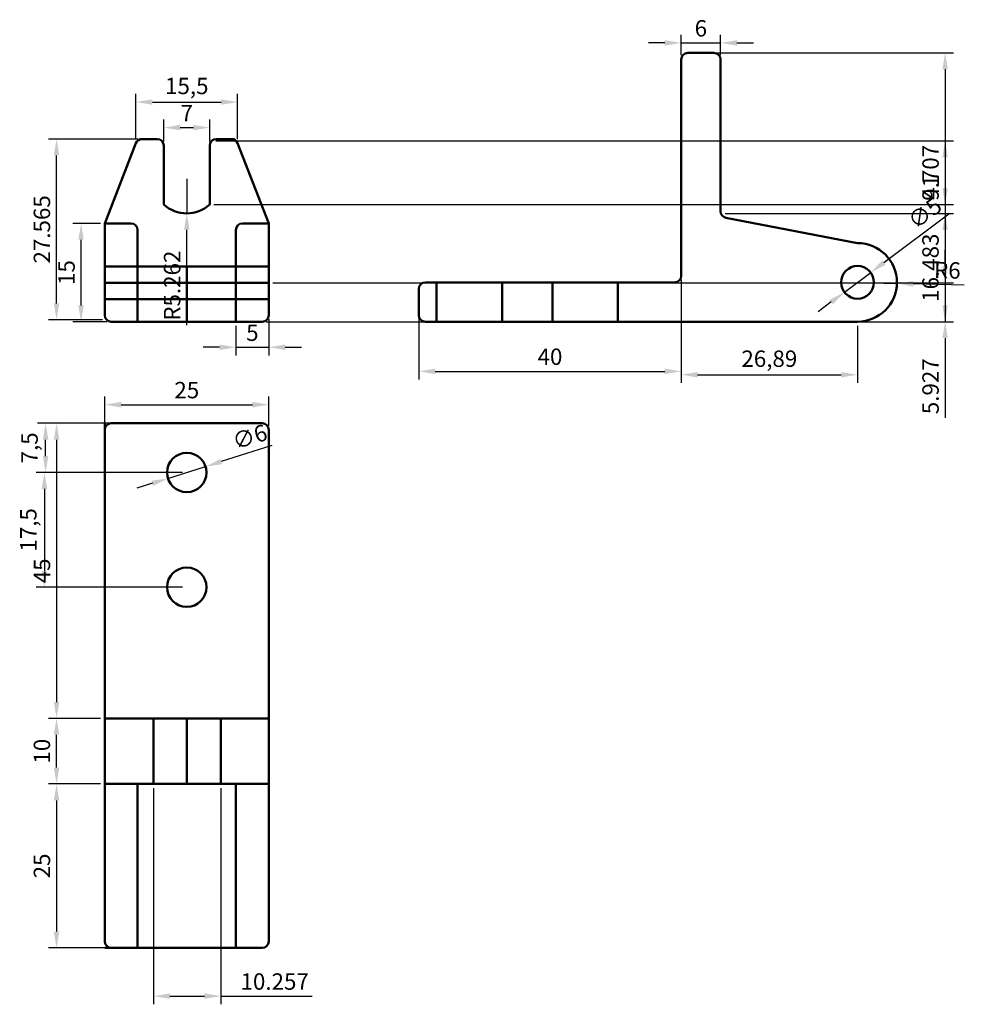
# Model space of a CAD drawing. Units: millimetres. Extents: x 2189 to 2333, y 2094 to 2245.
import ezdxf

# ---------------------------------------------------------------- set-up
doc = ezdxf.new("R2010")
doc.units = ezdxf.units.MM
doc.layers.add('M-DIMS', color=2, linetype='Continuous', lineweight=25)
doc.layers.add('M-OUTL', color=7, linetype='Continuous', lineweight=50)
doc.styles.get("Standard").update_dxf_attribs({"font": 'arial.ttf'})
doc.dimstyles.new('ISO-25', dxfattribs={"dimtxt": 2.5, "dimasz": 2.5, "dimexe": 1.25, "dimexo": 0.625, "dimtad": 1, "dimtxsty": 'Standard', "dimcen": 2.5, "dimadec": 0, "dimazin": 0, "dimtfac": 1, "dimtmove": 0, "dimatfit": 3, "dimfxl": 1, "dimarcsym": 0})

# ---------------------------------------------------------------- blocks, each defined once
blk = doc.blocks.new('*D1')
at = {"layer": 'Defpoints', "color": 0, "transparency": 16777216}
for p in [(2214.95, 2175.49), (2193.25, 2157.99), (2214.95, 2157.99)]:
    blk.add_point(p, dxfattribs=at)
at = {"layer": 'M-DIMS', "color": 0, "lineweight": -2, "transparency": 16777216}
for p, q in [((2214.32, 2175.49), (2192, 2175.49)), ((2193.25, 2172.99), (2193.25, 2160.49)), ((2214.32, 2157.99), (2192, 2157.99))]:
    blk.add_line(p, q, dxfattribs=at)
at = {"layer": 'M-DIMS', "color": 0, "transparency": 16777216}
for points in [[(2192.83, 2172.99), (2193.66, 2172.99), (2193.25, 2175.49)], [(2192.83, 2160.49), (2193.66, 2160.49), (2193.25, 2157.99)]]:
    blk.add_solid(points, dxfattribs=at)
at = {"layer": 'M-DIMS', "color": 0, "transparency": 16777216, "insert": (2191.12, 2166.74), "char_height": 2.5, "attachment_point": 5, "rotation": 90}
blk.add_mtext('17,5', dxfattribs=at)
blk = doc.blocks.new('*D2')
at = {"layer": 'Defpoints', "color": 0, "transparency": 16777216}
for p in [(2193.43, 2182.99), (2214.95, 2182.99), (2214.95, 2175.49)]:
    blk.add_point(p, dxfattribs=at)
at = {"layer": 'M-DIMS', "color": 0, "lineweight": -2, "transparency": 16777216}
for p, q in [((2214.32, 2182.99), (2192.18, 2182.99)), ((2193.43, 2177.99), (2193.43, 2180.49)), ((2214.32, 2175.49), (2192.18, 2175.49))]:
    blk.add_line(p, q, dxfattribs=at)
at = {"layer": 'M-DIMS', "color": 0, "transparency": 16777216}
for points in [[(2193.01, 2180.49), (2193.85, 2180.49), (2193.43, 2182.99)], [(2193.01, 2177.99), (2193.85, 2177.99), (2193.43, 2175.49)]]:
    blk.add_solid(points, dxfattribs=at)
at = {"layer": 'M-DIMS', "color": 0, "transparency": 16777216, "insert": (2191.31, 2179.24), "char_height": 2.5, "attachment_point": 5, "rotation": 90}
blk.add_mtext('7,5', dxfattribs=at)
blk = doc.blocks.new('*D3')
at = {"layer": 'Defpoints', "color": 0, "transparency": 16777216}
for p in [(2217.81, 2176.39), (2212.08, 2174.59)]:
    blk.add_point(p, dxfattribs=at)
at = {"layer": 'M-DIMS', "color": 0, "lineweight": -2, "transparency": 16777216}
for p, q in [((2227.92, 2179.59), (2220.19, 2177.15)), ((2212.08, 2174.59), (2217.81, 2176.39)), ((2209.7, 2173.84), (2207.32, 2173.08))]:
    blk.add_line(p, q, dxfattribs=at)
at = {"layer": 'M-DIMS', "color": 0, "transparency": 16777216}
for points in [[(2220.06, 2177.54), (2220.32, 2176.75), (2217.81, 2176.39)], [(2209.57, 2174.23), (2209.83, 2173.44), (2212.08, 2174.59)]]:
    blk.add_solid(points, dxfattribs=at)
at = {"layer": 'M-DIMS', "color": 0, "transparency": 16777216, "insert": (2224.65, 2180.62), "char_height": 2.5, "attachment_point": 5, "rotation": 17.516}
blk.add_mtext('∅6', dxfattribs=at)
blk = doc.blocks.new('*D4')
at = {"layer": 'Defpoints', "color": 0, "transparency": 16777216}
for p in [(2227.45, 2185.83), (2202.45, 2181.99), (2227.45, 2181.99)]:
    blk.add_point(p, dxfattribs=at)
at = {"layer": 'M-DIMS', "color": 0, "lineweight": -2, "transparency": 16777216}
for p, q in [((2202.45, 2182.62), (2202.45, 2187.08)), ((2227.45, 2182.62), (2227.45, 2187.08)), ((2204.95, 2185.83), (2224.95, 2185.83))]:
    blk.add_line(p, q, dxfattribs=at)
at = {"layer": 'M-DIMS', "color": 0, "transparency": 16777216}
for points in [[(2204.95, 2186.25), (2204.95, 2185.41), (2202.45, 2185.83)], [(2224.95, 2186.25), (2224.95, 2185.41), (2227.45, 2185.83)]]:
    blk.add_solid(points, dxfattribs=at)
at = {"layer": 'M-DIMS', "color": 0, "transparency": 16777216, "insert": (2214.95, 2187.73), "char_height": 2.5, "attachment_point": 5}
blk.add_mtext('25', dxfattribs=at)
blk = doc.blocks.new('*D5')
at = {"layer": 'Defpoints', "color": 0, "transparency": 16777216}
for p in [(2222.45, 2198.48), (2227.45, 2199.48), (2227.45, 2194.59)]:
    blk.add_point(p, dxfattribs=at)
at = {"layer": 'M-DIMS', "color": 0, "lineweight": -2, "transparency": 16777216}
for p, q in [((2227.45, 2198.86), (2227.45, 2193.34)), ((2222.45, 2197.86), (2222.45, 2193.34)), ((2219.95, 2194.59), (2217.45, 2194.59)), ((2222.45, 2194.59), (2227.45, 2194.59)), ((2229.95, 2194.59), (2232.45, 2194.59))]:
    blk.add_line(p, q, dxfattribs=at)
at = {"layer": 'M-DIMS', "color": 0, "transparency": 16777216}
for points in [[(2219.95, 2195), (2219.95, 2194.17), (2222.45, 2194.59)], [(2229.95, 2195), (2229.95, 2194.17), (2227.45, 2194.59)]]:
    blk.add_solid(points, dxfattribs=at)
at = {"layer": 'M-DIMS', "color": 0, "transparency": 16777216, "insert": (2224.95, 2196.48), "char_height": 2.5, "attachment_point": 5}
blk.add_mtext('5', dxfattribs=at)
blk = doc.blocks.new('*D6')
at = {"layer": 'Defpoints', "color": 0, "transparency": 16777216}
for p in [(2198.84, 2213.48), (2202.45, 2213.48), (2203.45, 2198.48)]:
    blk.add_point(p, dxfattribs=at)
at = {"layer": 'M-DIMS', "color": 0, "lineweight": -2, "transparency": 16777216}
for p, q in [((2201.82, 2213.48), (2197.59, 2213.48)), ((2198.84, 2200.98), (2198.84, 2210.98)), ((2202.82, 2198.48), (2197.59, 2198.48))]:
    blk.add_line(p, q, dxfattribs=at)
at = {"layer": 'M-DIMS', "color": 0, "transparency": 16777216}
for points in [[(2198.42, 2210.98), (2199.25, 2210.98), (2198.84, 2213.48)], [(2198.42, 2200.98), (2199.25, 2200.98), (2198.84, 2198.48)]]:
    blk.add_solid(points, dxfattribs=at)
at = {"layer": 'M-DIMS', "color": 0, "transparency": 16777216, "insert": (2196.94, 2205.98), "char_height": 2.5, "attachment_point": 5, "rotation": 90}
blk.add_mtext('15', dxfattribs=at)
blk = doc.blocks.new('*D7')
at = {"layer": 'Defpoints', "color": 0, "transparency": 16777216}
for p in [(2218.45, 2228.08), (2211.45, 2225.34), (2218.45, 2225.34)]:
    blk.add_point(p, dxfattribs=at)
at = {"layer": 'M-DIMS', "color": 0, "lineweight": -2, "transparency": 16777216}
for p, q in [((2211.45, 2225.97), (2211.45, 2229.33)), ((2218.45, 2225.97), (2218.45, 2229.33)), ((2213.95, 2228.08), (2215.95, 2228.08))]:
    blk.add_line(p, q, dxfattribs=at)
at = {"layer": 'M-DIMS', "color": 0, "transparency": 16777216}
for points in [[(2213.95, 2228.5), (2213.95, 2227.67), (2211.45, 2228.08)], [(2215.95, 2228.5), (2215.95, 2227.67), (2218.45, 2228.08)]]:
    blk.add_solid(points, dxfattribs=at)
at = {"layer": 'M-DIMS', "color": 0, "transparency": 16777216, "insert": (2214.95, 2229.96), "char_height": 2.5, "attachment_point": 5}
blk.add_mtext('7', dxfattribs=at)
blk = doc.blocks.new('*D8')
at = {"layer": 'Defpoints', "color": 0, "transparency": 16777216}
for p in [(2222.69, 2231.98), (2207.2, 2225.7), (2222.69, 2225.7)]:
    blk.add_point(p, dxfattribs=at)
at = {"layer": 'M-DIMS', "color": 0, "lineweight": -2, "transparency": 16777216}
for p, q in [((2207.2, 2226.33), (2207.2, 2233.23)), ((2222.69, 2226.33), (2222.69, 2233.23)), ((2209.7, 2231.98), (2220.19, 2231.98))]:
    blk.add_line(p, q, dxfattribs=at)
at = {"layer": 'M-DIMS', "color": 0, "transparency": 16777216}
for points in [[(2209.7, 2232.39), (2209.7, 2231.56), (2207.2, 2231.98)], [(2220.19, 2232.39), (2220.19, 2231.56), (2222.69, 2231.98)]]:
    blk.add_solid(points, dxfattribs=at)
at = {"layer": 'M-DIMS', "color": 0, "transparency": 16777216, "insert": (2214.95, 2234.11), "char_height": 2.5, "attachment_point": 5}
blk.add_mtext('15,5', dxfattribs=at)
blk = doc.blocks.new('*D9')
at = {"layer": 'Defpoints', "color": 0, "transparency": 16777216}
for p in [(2296.32, 2241), (2290.32, 2238.48), (2296.32, 2238.48)]:
    blk.add_point(p, dxfattribs=at)
at = {"layer": 'M-DIMS', "color": 0, "lineweight": -2, "transparency": 16777216}
for p, q in [((2290.32, 2239.11), (2290.32, 2242.25)), ((2296.32, 2239.11), (2296.32, 2242.25)), ((2287.82, 2241), (2285.32, 2241)), ((2290.32, 2241), (2296.32, 2241)), ((2298.82, 2241), (2301.32, 2241))]:
    blk.add_line(p, q, dxfattribs=at)
at = {"layer": 'M-DIMS', "color": 0, "transparency": 16777216}
for points in [[(2287.82, 2241.41), (2287.82, 2240.58), (2290.32, 2241)], [(2298.82, 2241.41), (2298.82, 2240.58), (2296.32, 2241)]]:
    blk.add_solid(points, dxfattribs=at)
at = {"layer": 'M-DIMS', "color": 0, "transparency": 16777216, "insert": (2293.32, 2242.9), "char_height": 2.5, "attachment_point": 5}
blk.add_mtext('6', dxfattribs=at)
blk = doc.blocks.new('*D10')
at = {"layer": 'Defpoints', "color": 0, "transparency": 16777216}
for p in [(2319.21, 2205.98), (2315.21, 2202.98)]:
    blk.add_point(p, dxfattribs=at)
at = {"layer": 'M-DIMS', "color": 0, "lineweight": -2, "transparency": 16777216}
for p, q in [((2331.1, 2214.89), (2321.21, 2207.48)), ((2315.21, 2202.98), (2319.21, 2205.98)), ((2313.2, 2201.49), (2311.2, 2199.99))]:
    blk.add_line(p, q, dxfattribs=at)
at = {"layer": 'M-DIMS', "color": 0, "transparency": 16777216}
for points in [[(2320.96, 2207.81), (2321.46, 2207.15), (2319.21, 2205.98)], [(2312.95, 2201.82), (2313.45, 2201.15), (2315.21, 2202.98)]]:
    blk.add_solid(points, dxfattribs=at)
at = {"layer": 'M-DIMS', "color": 0, "transparency": 16777216, "insert": (2327.66, 2214.78), "char_height": 2.5, "attachment_point": 5, "rotation": 36.8282}
blk.add_mtext('∅5', dxfattribs=at)
blk = doc.blocks.new('*D11')
at = {"layer": 'Defpoints', "color": 0, "transparency": 16777216}
for p in [(2290.32, 2205.48), (2250.32, 2203.48), (2290.32, 2190.91)]:
    blk.add_point(p, dxfattribs=at)
at = {"layer": 'M-DIMS', "color": 0, "lineweight": -2, "transparency": 16777216}
for p, q in [((2290.32, 2204.86), (2290.32, 2189.66)), ((2250.32, 2202.86), (2250.32, 2189.66)), ((2252.82, 2190.91), (2287.82, 2190.91))]:
    blk.add_line(p, q, dxfattribs=at)
at = {"layer": 'M-DIMS', "color": 0, "transparency": 16777216}
for points in [[(2252.82, 2191.33), (2252.82, 2190.5), (2250.32, 2190.91)], [(2287.82, 2191.33), (2287.82, 2190.5), (2290.32, 2190.91)]]:
    blk.add_solid(points, dxfattribs=at)
at = {"layer": 'M-DIMS', "color": 0, "transparency": 16777216, "insert": (2270.32, 2192.82), "char_height": 2.5, "attachment_point": 5}
blk.add_mtext('40', dxfattribs=at)
blk = doc.blocks.new('*D12')
at = {"layer": 'Defpoints', "color": 0, "transparency": 16777216}
for p in [(2317.21, 2198.48), (2290.32, 2197.26), (2317.21, 2190.4)]:
    blk.add_point(p, dxfattribs=at)
at = {"layer": 'M-DIMS', "color": 0, "lineweight": -2, "transparency": 16777216}
for p, q in [((2317.21, 2197.86), (2317.21, 2189.15)), ((2290.32, 2196.64), (2290.32, 2189.15)), ((2292.82, 2190.4), (2314.71, 2190.4))]:
    blk.add_line(p, q, dxfattribs=at)
at = {"layer": 'M-DIMS', "color": 0, "transparency": 16777216}
for points in [[(2292.82, 2190.81), (2292.82, 2189.98), (2290.32, 2190.4)], [(2314.71, 2190.81), (2314.71, 2189.98), (2317.21, 2190.4)]]:
    blk.add_solid(points, dxfattribs=at)
at = {"layer": 'M-DIMS', "color": 0, "transparency": 16777216, "insert": (2303.76, 2192.52), "char_height": 2.5, "attachment_point": 5}
blk.add_mtext('26,89', dxfattribs=at)
blk = doc.blocks.new('*D13')
at = {"layer": 'Defpoints', "color": 0, "transparency": 16777216}
for p in [(2317.21, 2204.48), (2323.2, 2204.32)]:
    blk.add_point(p, dxfattribs=at)
at = {"layer": 'M-DIMS', "color": 0, "lineweight": -2, "transparency": 16777216}
for p, q in [((2317.21, 2204.48), (2323.2, 2204.32)), ((2333.48, 2204.04), (2325.7, 2204.25))]:
    blk.add_line(p, q, dxfattribs=at)
at = {"layer": 'M-DIMS', "color": 0, "transparency": 16777216}
blk.add_solid([(2325.71, 2204.67), (2325.69, 2203.83), (2323.2, 2204.32)], dxfattribs=at)
at = {"layer": 'M-DIMS', "color": 0, "transparency": 16777216, "insert": (2330.89, 2206.01), "char_height": 2.5, "attachment_point": 5, "rotation": 358.4247}
blk.add_mtext('R6', dxfattribs=at)
blk = doc.blocks.new('*D14')
at = {"layer": 'Defpoints', "color": 0, "transparency": 16777216}
for p in [(2291.32, 2239.48), (2317.21, 2198.48), (2330.56, 2198.48)]:
    blk.add_point(p, dxfattribs=at)
at = {"layer": 'M-DIMS', "color": 0, "lineweight": -2, "transparency": 16777216}
for p, q in [((2291.95, 2239.48), (2331.81, 2239.48)), ((2330.56, 2236.98), (2330.56, 2200.98)), ((2317.83, 2198.48), (2331.81, 2198.48))]:
    blk.add_line(p, q, dxfattribs=at)
at = {"layer": 'M-DIMS', "color": 0, "transparency": 16777216}
for points in [[(2330.14, 2236.98), (2330.97, 2236.98), (2330.56, 2239.48)], [(2330.14, 2200.98), (2330.97, 2200.98), (2330.56, 2198.48)]]:
    blk.add_solid(points, dxfattribs=at)
at = {"layer": 'M-DIMS', "color": 0, "transparency": 16777216, "insert": (2328.68, 2218.98), "char_height": 2.5, "attachment_point": 5, "rotation": 90}
blk.add_mtext('41', dxfattribs=at)
blk = doc.blocks.new('*D15')
at = {"layer": 'Defpoints', "color": 0, "transparency": 16777216}
for p in [(2227.45, 2204.41), (2226.45, 2198.48), (2330.56, 2198.48)]:
    blk.add_point(p, dxfattribs=at)
at = {"layer": 'M-DIMS', "color": 0, "lineweight": -2, "transparency": 16777216}
for p, q in [((2330.56, 2206.91), (2330.56, 2209.41)), ((2228.07, 2204.41), (2331.81, 2204.41)), ((2330.56, 2204.41), (2330.56, 2198.48)), ((2227.07, 2198.48), (2331.81, 2198.48)), ((2330.56, 2195.98), (2330.56, 2183.8))]:
    blk.add_line(p, q, dxfattribs=at)
at = {"layer": 'M-DIMS', "color": 0, "transparency": 16777216}
for points in [[(2330.14, 2206.91), (2330.97, 2206.91), (2330.56, 2204.41)], [(2330.14, 2195.98), (2330.97, 2195.98), (2330.56, 2198.48)]]:
    blk.add_solid(points, dxfattribs=at)
at = {"layer": 'M-DIMS', "color": 0, "transparency": 16777216, "insert": (2328.66, 2188.64), "char_height": 2.5, "attachment_point": 5, "rotation": 90}
blk.add_mtext('5.927', dxfattribs=at)
blk = doc.blocks.new('*D16')
at = {"layer": 'Defpoints', "color": 0, "transparency": 16777216}
for p in [(2296.38, 2214.97), (2297.32, 2198.48), (2330.56, 2198.48)]:
    blk.add_point(p, dxfattribs=at)
at = {"layer": 'M-DIMS', "color": 0, "lineweight": -2, "transparency": 16777216}
for p, q in [((2297.01, 2214.97), (2331.81, 2214.97)), ((2330.56, 2212.47), (2330.56, 2200.98)), ((2297.95, 2198.48), (2331.81, 2198.48))]:
    blk.add_line(p, q, dxfattribs=at)
at = {"layer": 'M-DIMS', "color": 0, "transparency": 16777216}
for points in [[(2330.14, 2212.47), (2330.97, 2212.47), (2330.56, 2214.97)], [(2330.14, 2200.98), (2330.97, 2200.98), (2330.56, 2198.48)]]:
    blk.add_solid(points, dxfattribs=at)
at = {"layer": 'M-DIMS', "color": 0, "transparency": 16777216, "insert": (2328.65, 2206.72), "char_height": 2.5, "attachment_point": 5, "rotation": 90}
blk.add_mtext('16.483', dxfattribs=at)
blk = doc.blocks.new('*D17')
at = {"layer": 'Defpoints', "color": 0, "transparency": 16777216}
for p in [(2195.1, 2226.34), (2208.13, 2226.34), (2202.74, 2198.78)]:
    blk.add_point(p, dxfattribs=at)
at = {"layer": 'M-DIMS', "color": 0, "lineweight": -2, "transparency": 16777216}
for p, q in [((2207.5, 2226.34), (2193.85, 2226.34)), ((2195.1, 2201.28), (2195.1, 2223.84)), ((2202.11, 2198.78), (2193.85, 2198.78))]:
    blk.add_line(p, q, dxfattribs=at)
at = {"layer": 'M-DIMS', "color": 0, "transparency": 16777216}
for points in [[(2194.68, 2223.84), (2195.51, 2223.84), (2195.1, 2226.34)], [(2194.68, 2201.28), (2195.51, 2201.28), (2195.1, 2198.78)]]:
    blk.add_solid(points, dxfattribs=at)
at = {"layer": 'M-DIMS', "color": 0, "transparency": 16777216, "insert": (2193.19, 2212.56), "char_height": 2.5, "attachment_point": 5, "rotation": 90}
blk.add_mtext('27.565', dxfattribs=at)
blk = doc.blocks.new('*D18')
at = {"layer": 'Defpoints', "color": 0, "transparency": 16777216}
for p in [(2218.74, 2226.05), (2218.45, 2216.34), (2330.56, 2216.34)]:
    blk.add_point(p, dxfattribs=at)
at = {"layer": 'M-DIMS', "color": 0, "lineweight": -2, "transparency": 16777216}
for p, q in [((2219.36, 2226.05), (2331.81, 2226.05)), ((2330.56, 2223.55), (2330.56, 2218.84)), ((2219.07, 2216.34), (2331.81, 2216.34))]:
    blk.add_line(p, q, dxfattribs=at)
at = {"layer": 'M-DIMS', "color": 0, "transparency": 16777216}
for points in [[(2330.14, 2223.55), (2330.97, 2223.55), (2330.56, 2226.05)], [(2330.14, 2218.84), (2330.97, 2218.84), (2330.56, 2216.34)]]:
    blk.add_solid(points, dxfattribs=at)
at = {"layer": 'M-DIMS', "color": 0, "transparency": 16777216, "insert": (2328.66, 2221.19), "char_height": 2.5, "attachment_point": 5, "rotation": 90}
blk.add_mtext('9.707', dxfattribs=at)
blk = doc.blocks.new('*D19')
at = {"layer": 'Defpoints', "color": 0, "transparency": 16777216}
for p in [(2203.45, 2182.99), (2195.1, 2137.99), (2202.45, 2137.99)]:
    blk.add_point(p, dxfattribs=at)
at = {"layer": 'M-DIMS', "color": 0, "lineweight": -2, "transparency": 16777216}
for p, q in [((2202.82, 2182.99), (2193.85, 2182.99)), ((2195.1, 2180.49), (2195.1, 2140.49)), ((2201.82, 2137.99), (2193.85, 2137.99))]:
    blk.add_line(p, q, dxfattribs=at)
at = {"layer": 'M-DIMS', "color": 0, "transparency": 16777216}
for points in [[(2194.68, 2180.49), (2195.51, 2180.49), (2195.1, 2182.99)], [(2194.68, 2140.49), (2195.51, 2140.49), (2195.1, 2137.99)]]:
    blk.add_solid(points, dxfattribs=at)
at = {"layer": 'M-DIMS', "color": 0, "transparency": 16777216, "insert": (2193.2, 2160.49), "char_height": 2.5, "attachment_point": 5, "rotation": 90}
blk.add_mtext('45', dxfattribs=at)
blk = doc.blocks.new('*D20')
at = {"layer": 'Defpoints', "color": 0, "transparency": 16777216}
for p in [(2202.45, 2127.99), (2195.1, 2102.99), (2203.45, 2102.99)]:
    blk.add_point(p, dxfattribs=at)
at = {"layer": 'M-DIMS', "color": 0, "lineweight": -2, "transparency": 16777216}
for p, q in [((2201.82, 2127.99), (2193.85, 2127.99)), ((2195.1, 2125.49), (2195.1, 2105.49)), ((2202.82, 2102.99), (2193.85, 2102.99))]:
    blk.add_line(p, q, dxfattribs=at)
at = {"layer": 'M-DIMS', "color": 0, "transparency": 16777216}
for points in [[(2194.68, 2125.49), (2195.51, 2125.49), (2195.1, 2127.99)], [(2194.68, 2105.49), (2195.51, 2105.49), (2195.1, 2102.99)]]:
    blk.add_solid(points, dxfattribs=at)
at = {"layer": 'M-DIMS', "color": 0, "transparency": 16777216, "insert": (2193.19, 2115.49), "char_height": 2.5, "attachment_point": 5, "rotation": 90}
blk.add_mtext('25', dxfattribs=at)
blk = doc.blocks.new('*D21')
at = {"layer": 'Defpoints', "color": 0, "transparency": 16777216}
for p in [(2195.1, 2137.99), (2202.45, 2137.99), (2202.45, 2127.99)]:
    blk.add_point(p, dxfattribs=at)
at = {"layer": 'M-DIMS', "color": 0, "lineweight": -2, "transparency": 16777216}
for p, q in [((2201.82, 2137.99), (2193.85, 2137.99)), ((2195.1, 2130.49), (2195.1, 2135.49)), ((2201.82, 2127.99), (2193.85, 2127.99))]:
    blk.add_line(p, q, dxfattribs=at)
at = {"layer": 'M-DIMS', "color": 0, "transparency": 16777216}
for points in [[(2194.68, 2135.49), (2195.51, 2135.49), (2195.1, 2137.99)], [(2194.68, 2130.49), (2195.51, 2130.49), (2195.1, 2127.99)]]:
    blk.add_solid(points, dxfattribs=at)
at = {"layer": 'M-DIMS', "color": 0, "transparency": 16777216, "insert": (2193.19, 2132.99), "char_height": 2.5, "attachment_point": 5, "rotation": 90}
blk.add_mtext('10', dxfattribs=at)
blk = doc.blocks.new('*D22')
at = {"layer": 'Defpoints', "color": 0, "transparency": 16777216}
for p in [(2209.89, 2127.99), (2220.15, 2127.99), (2220.15, 2095.64)]:
    blk.add_point(p, dxfattribs=at)
at = {"layer": 'M-DIMS', "color": 0, "lineweight": -2, "transparency": 16777216}
for p, q in [((2209.89, 2127.37), (2209.89, 2094.39)), ((2220.15, 2127.37), (2220.15, 2094.39)), ((2212.39, 2095.64), (2217.65, 2095.64)), ((2220.15, 2095.64), (2234.04, 2095.64))]:
    blk.add_line(p, q, dxfattribs=at)
at = {"layer": 'M-DIMS', "color": 0, "transparency": 16777216}
for points in [[(2212.39, 2096.06), (2212.39, 2095.22), (2209.89, 2095.64)], [(2217.65, 2096.06), (2217.65, 2095.22), (2220.15, 2095.64)]]:
    blk.add_solid(points, dxfattribs=at)
at = {"layer": 'M-DIMS', "color": 0, "transparency": 16777216, "insert": (2228.35, 2097.54), "char_height": 2.5, "attachment_point": 5}
blk.add_mtext('10.257', dxfattribs=at)
blk = doc.blocks.new('*D23')
at = {"layer": 'Defpoints', "color": 0, "transparency": 16777216}
for p in [(2214.95, 2220.27), (2214.95, 2215.01)]:
    blk.add_point(p, dxfattribs=at)
at = {"layer": 'M-DIMS', "color": 0, "lineweight": -2, "transparency": 16777216}
for p, q in [((2214.95, 2220.27), (2214.95, 2215.01)), ((2214.94, 2197.96), (2214.94, 2212.51))]:
    blk.add_line(p, q, dxfattribs=at)
at = {"layer": 'M-DIMS', "color": 0, "transparency": 16777216}
blk.add_solid([(2214.53, 2212.51), (2215.36, 2212.51), (2214.95, 2215.01)], dxfattribs=at)
at = {"layer": 'M-DIMS', "color": 0, "transparency": 16777216, "insert": (2213.04, 2203.98), "char_height": 2.5, "attachment_point": 5, "rotation": 89.9962}
blk.add_mtext('R5.262', dxfattribs=at)

msp = doc.modelspace()

# ---------------------------------------------------------------- linework, layer by layer
at = {"layer": 'M-OUTL'}
for p, q in [((2291.3215, 2239.483), (2295.3215, 2239.483)), ((2290.3215, 2205.483), (2290.3215, 2238.483)), ((2296.3215, 2238.483), (2296.3215, 2215.3096)), ((2207.1974, 2225.7038), (2202.4453, 2213.483)), ((2210.4453, 2226.3414), (2208.1294, 2226.3414)), ((2211.4453, 2216.3414), (2211.4453, 2225.3414)), ((2218.4453, 2225.3414), (2218.4453, 2216.3414)), ((2219.4453, 2226.3414), (2221.7613, 2226.3414)), ((2222.6933, 2225.7038), (2227.4453, 2213.483)), ((2202.4453, 2199.483), (2202.4453, 2213.483)), ((2202.4453, 2213.483), (2206.4453, 2213.483)), ((2227.4453, 2213.483), (2223.4453, 2213.483)), ((2227.4453, 2199.483), (2227.4453, 2213.483)), ((2297.1334, 2214.3275), (2317.2067, 2210.483)), ((2207.4453, 2198.483), (2207.4453, 2212.483)), ((2222.4453, 2212.483), (2222.4453, 2198.483)), ((2227.4453, 2206.9096), (2202.4453, 2206.9096)), ((2214.9453, 2198.483), (2214.9453, 2206.9096)), ((2202.4453, 2204.4096), (2227.4453, 2204.4096)), ((2251.3215, 2204.483), (2289.3215, 2204.483)), ((2253.0404, 2204.483), (2253.0404, 2198.483)), ((2263.0404, 2204.483), (2263.0404, 2198.483)), ((2270.6856, 2204.483), (2270.6856, 2198.483)), ((2280.6856, 2204.483), (2280.6856, 2198.483)), ((2250.3215, 2199.483), (2250.3215, 2203.483)), ((2202.4453, 2201.9096), (2227.4453, 2201.9096)), ((2203.4453, 2198.483), (2226.4453, 2198.483)), ((2251.3215, 2198.483), (2297.3215, 2198.483)), ((2297.3215, 2198.483), (2317.2067, 2198.483)), ((2202.4453, 2103.9912), (2202.4453, 2182.9912)), ((2202.4453, 2181.9912), (2202.4453, 2175.4912)), ((2203.4453, 2182.9912), (2226.4453, 2182.9912)), ((2227.4453, 2181.9912), (2227.4453, 2103.9912)), ((2202.4453, 2175.4912), (2202.4453, 2157.9912)), ((2202.4453, 2137.9912), (2227.4453, 2137.9912)), ((2209.8938, 2137.9912), (2209.8938, 2127.9912)), ((2214.9453, 2137.9912), (2214.9453, 2127.9912)), ((2220.1507, 2137.9912), (2220.1507, 2127.9912)), ((2207.4453, 2127.9912), (2202.4453, 2127.9912)), ((2207.4453, 2102.9912), (2207.4453, 2127.9912)), ((2207.4453, 2127.9912), (2222.4453, 2127.9912)), ((2222.4453, 2127.9912), (2222.4453, 2102.9912)), ((2227.4453, 2127.9912), (2222.4453, 2127.9912)), ((2226.4453, 2102.9912), (2202.4453, 2102.9912)), ((2203.4453, 2102.9912), (2207.4453, 2102.9912))]:
    msp.add_line(p, q, dxfattribs=at)
for centre, radius in [((2317.2067, 2204.483), 2.5), ((2214.9453, 2175.4912), 3), ((2214.9453, 2157.9912), 3)]:
    msp.add_circle(centre, radius, dxfattribs=at)
for centre, radius, start, end in [((2291.3215, 2238.483), 1, 90, 180), ((2295.3215, 2238.483), 1, 0, 90), ((2208.1294, 2225.3414), 1, 90, 158.751358), ((2210.4453, 2225.3414), 1, 0, 90), ((2219.4453, 2225.3414), 1, 90, 180), ((2221.7613, 2225.3414), 1, 21.248642, 90), ((2214.9453, 2220.2706), 5.262, 228.306349, 311.693651), ((2297.3215, 2215.3096), 1, 180, 259.157821), ((2206.4453, 2212.483), 1, 0, 90), ((2223.4453, 2212.483), 1, 90, 180), ((2317.2067, 2204.483), 6, 270, 90), ((2251.3215, 2203.483), 1, 90, 180), ((2289.3215, 2205.483), 1, 270, 0), ((2203.4453, 2199.483), 1, 180, 270), ((2226.4453, 2199.483), 1, 270, 0), ((2251.3215, 2199.483), 1, 180, 270), ((2203.4453, 2181.9912), 1, 90, 180), ((2226.4453, 2181.9912), 1, 0, 90), ((2203.4453, 2103.9912), 1, 180, 270), ((2226.4453, 2103.9912), 1, 270, 0)]:
    msp.add_arc(centre, radius, start, end, dxfattribs=at)

# ---------------------------------------------------------------- dimensions: what is measured, and where the dimension line sits
at = {"layer": 'M-DIMS'}
for base, p1, p2, override, picture, middle in [((2296.3215, 2240.9974), (2290.3215, 2238.483), (2296.3215, 2238.483), {"dimclrd": 0, "dimclre": 0, "dimclrt": 0}, '*D9', (2293.3215, 2242.8989)), ((2222.6933, 2231.9781), (2207.1974, 2225.7038), (2222.6933, 2225.7038), {"dimclrd": 0, "dimclre": 0, "dimclrt": 0}, '*D8', (2214.9453, 2234.1054)), ((2218.4453, 2228.0834), (2211.4453, 2225.3414), (2218.4453, 2225.3414), {"dimclrd": 0, "dimclre": 0, "dimclrt": 0}, '*D7', (2214.9453, 2229.9584)), ((2290.3215, 2190.9141), (2250.3215, 2203.483), (2290.3215, 2205.483), {"dimclrd": 0, "dimclre": 0, "dimclrt": 0}, '*D11', (2270.3215, 2192.8156)), ((2227.4453, 2194.5854), (2222.4453, 2198.483), (2227.4453, 2199.483), {"dimclrd": 0, "dimclre": 0, "dimclrt": 0}, '*D5', (2224.9453, 2196.4817)), ((2317.2067, 2190.3955), (2290.3215, 2197.2611), (2317.2067, 2198.483), {"dimclrd": 0, "dimclre": 0, "dimclrt": 0}, '*D12', (2303.7641, 2192.5229)), ((2227.4453, 2185.8299), (2202.4453, 2181.9912), (2227.4453, 2181.9912), {"dimclrd": 0, "dimclre": 0, "dimclrt": 0}, '*D4', (2214.9453, 2187.7313)), ((2220.1507, 2095.6412), (2209.8938, 2127.9912), (2220.1507, 2127.9912), {"dimdec": 3, "dimlfac": 1, "dimrnd": 0, "dimzin": 0, "dimdsep": 46, "dimlunit": 2}, '*D22', (2228.3474, 2097.5426))]:
    dim = msp.add_linear_dim(base=base, p1=p1, p2=p2, dimstyle='ISO-25', override=override, dxfattribs=at)
    dim.commit()
    dim.dimension.update_dxf_attribs({"geometry": picture, "text_midpoint": middle})
for base, p1, p2, override, picture, middle in [((2330.5567, 2198.483), (2291.3215, 2239.483), (2317.2067, 2198.483), {"dimdec": 0, "dimlfac": 1, "dimrnd": 0, "dimzin": 0, "dimdsep": 46, "dimlunit": 2}, '*D14', (2328.6766, 2218.983)), ((2195.09535, 2226.34137), (2202.73824, 2198.77589), (2208.12944, 2226.34137), {"dimdec": 3, "dimlfac": 1, "dimrnd": 0, "dimzin": 0, "dimdsep": 46, "dimlunit": 2}, '*D17', (2193.19392, 2212.55863)), ((2330.5567, 2216.3414), (2218.7382, 2226.0485), (2218.4453, 2216.3414), {"dimdec": 3, "dimlfac": 1, "dimrnd": 0, "dimzin": 0, "dimdsep": 46, "dimlunit": 2}, '*D18', (2328.6553, 2221.1949)), ((2330.5567, 2198.48299), (2296.38211, 2214.96648), (2297.32151, 2198.48299), {"dimdec": 3, "dimlfac": 1, "dimrnd": 0, "dimzin": 0, "dimdsep": 46, "dimlunit": 2}, '*D16', (2328.65442, 2206.72474)), ((2198.8368, 2213.483), (2203.4453, 2198.483), (2202.4453, 2213.483), {"dimclrd": 0, "dimclre": 0, "dimclrt": 0}, '*D6', (2196.9354, 2205.983)), ((2330.5567, 2198.483), (2227.4453, 2204.4096), (2226.4453, 2198.483), {"dimdec": 3, "dimlfac": 1, "dimrnd": 0, "dimzin": 0, "dimdsep": 46, "dimlunit": 2}, '*D15', (2328.6553, 2188.6399)), ((2193.4301, 2182.9912), (2214.9453, 2175.4912), (2214.9453, 2182.9912), {"dimclrd": 0, "dimclre": 0, "dimclrt": 0}, '*D2', (2191.3078, 2179.2412)), ((2195.0953, 2137.9912), (2203.4453, 2182.9912), (2202.4453, 2137.9912), {"dimdec": 0, "dimlfac": 1, "dimrnd": 0, "dimzin": 0, "dimdsep": 46, "dimlunit": 2}, '*D19', (2193.199, 2160.4912)), ((2193.2467, 2157.9912), (2214.9453, 2175.4912), (2214.9453, 2157.9912), {"dimclrd": 0, "dimclre": 0, "dimclrt": 0}, '*D1', (2191.1193, 2166.7412)), ((2195.0953, 2137.9912), (2202.4453, 2127.9912), (2202.4453, 2137.9912), {"dimdec": 0, "dimlfac": 1, "dimrnd": 0, "dimzin": 0, "dimdsep": 46, "dimlunit": 2}, '*D21', (2193.1939, 2132.9912)), ((2195.0953, 2102.9912), (2202.4453, 2127.9912), (2203.4453, 2102.9912), {"dimdec": 0, "dimlfac": 1, "dimrnd": 0, "dimzin": 0, "dimdsep": 46, "dimlunit": 2}, '*D20', (2193.1939, 2115.4912))]:
    dim = msp.add_linear_dim(base=base, p1=p1, p2=p2, angle=90, dimstyle='ISO-25', override=override, dxfattribs=at)
    dim.commit()
    dim.dimension.update_dxf_attribs({"geometry": picture, "text_midpoint": middle})
for center, mpoint, override, picture, middle in [((2214.9453, 2220.2706), (2214.945, 2215.0086), {"dimdec": 3, "dimlfac": 1, "dimrnd": 0, "dimzin": 0, "dimdsep": 46, "dimlunit": 2}, '*D23', (2213.0428, 2203.9821)), ((2317.2067, 2204.483), (2323.2044, 2204.318), {"dimclrd": 0, "dimclre": 0, "dimclrt": 0}, '*D13', (2330.8937, 2206.0087))]:
    dim = msp.add_radius_dim(center=center, mpoint=mpoint, dimstyle='ISO-25', override=override, dxfattribs=at)
    dim.commit()
    dim.dimension.update_dxf_attribs({"geometry": picture, "text_midpoint": middle})
dim = msp.add_diameter_dim_2p(p1=(2315.2056, 2202.9844), p2=(2319.2078, 2205.9815), dimstyle='ISO-25', override={"dimclrd": 0, "dimclre": 0, "dimclrt": 0}, dxfattribs=at)
dim.commit()
dim.dimension.update_dxf_attribs({"geometry": '*D10', "text_midpoint": (2328.8461, 2213.1993), "dimtype": 163})
dim = msp.add_diameter_dim_2p(p1=(2212.0844, 2174.5883), p2=(2217.8062, 2176.3941), dimstyle='ISO-25', override={"dimclrd": 0, "dimclre": 0, "dimclrt": 0}, dxfattribs=at)
dim.commit()
dim.dimension.update_dxf_attribs({"geometry": '*D3', "text_midpoint": (2224.6546, 2180.6227)})

doc.saveas('drawing.dxf')
